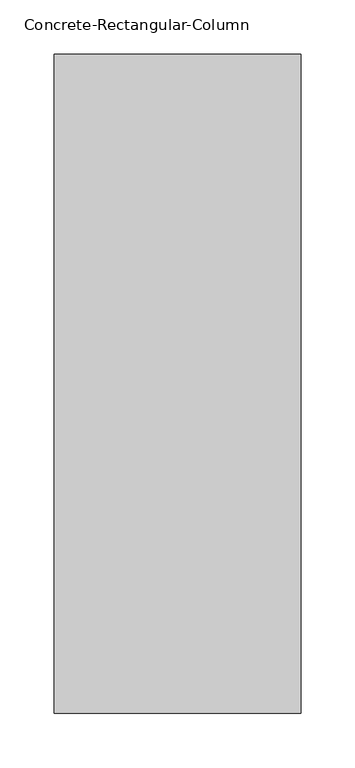
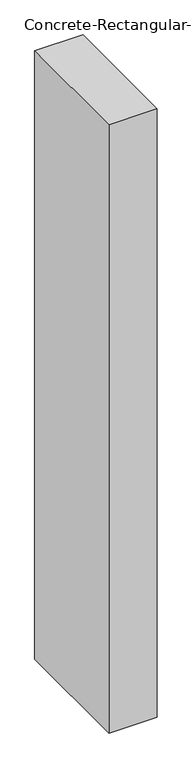
"""IFC4 building model written with IfcOpenShell, lengths in millimetres: column geometry, Concrete-Rectangular-Column."""

from ifc_helpers import new_model, si_unit, origin, origin_with_axes, place, context, project, spatial, polyline, outline, extrude, source, transform, mapped, element, save


def concrete_rectangular_column_147977c2(model_context):
    return source(origin(), model_context, "Body", "SweptSolid", [
        extrude(outline(polyline([(114.3, 304.8), (114.3, -304.8), (-114.3, -304.8), (-114.3, 304.8), (114.3, 304.8)])), origin_with_axes(), (0.0, 0.0, 1.0), 3048.0),
    ])


if __name__ == "__main__":
    model = new_model("IFC4")
    model_context = context("Model", 3, world=origin())
    ifc_project = project(units=[si_unit("LENGTHUNIT", "METRE", prefix="MILLI")], contexts=[model_context])
    site = spatial("IfcSite", under=ifc_project)
    building = spatial("IfcBuilding", under=site)
    placement = place(None, origin())
    concrete_rectangular_column_shape = concrete_rectangular_column_147977c2(model_context)
    element("IfcColumn", 1, ObjectType="Concrete-Rectangular-Column", at=placement, inside=building, context=model_context, shape_type="MappedRepresentation", body=[
        mapped(concrete_rectangular_column_shape, transform((0.0, 0.0, 0.0), x_axis=(1.0, 0.0, 0.0), y_axis=(0.0, 1.0, 0.0), z_axis=(0.0, 0.0, 1.0))),
    ])
    save(model, "model.ifc")

# Revit data of these elements
# Type "Concrete-Rectangular-Column"
#   Assembly Code = "B10"
#   b = 0' - 9"
#   h = 2' - 0"
#   Structural Material [instance default] = Concrete, Cast-in-Place gray
# Element 1 (IfcColumn, "Concrete-Rectangular-Column")
#   Structural Material = Concrete
#   Materials on its faces: "Concrete"
# Materials
#   "Concrete, Cast-in-Place gray": class "Concrete", colour RGB 192 192 192, transparency 0, Description = "Cast-in-place concrete", Cost = 0
#   "Concrete": class "Concrete", colour RGB 120 120 120, transparency 0, Description = "Portland Cement Concrete", Cost = 0
